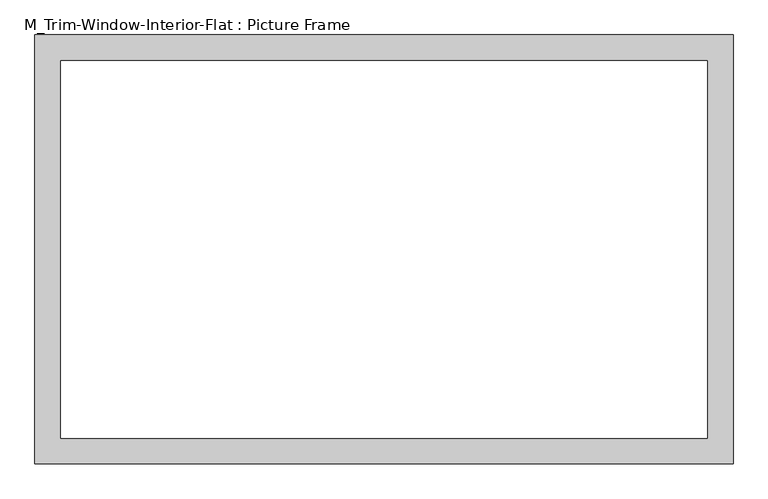
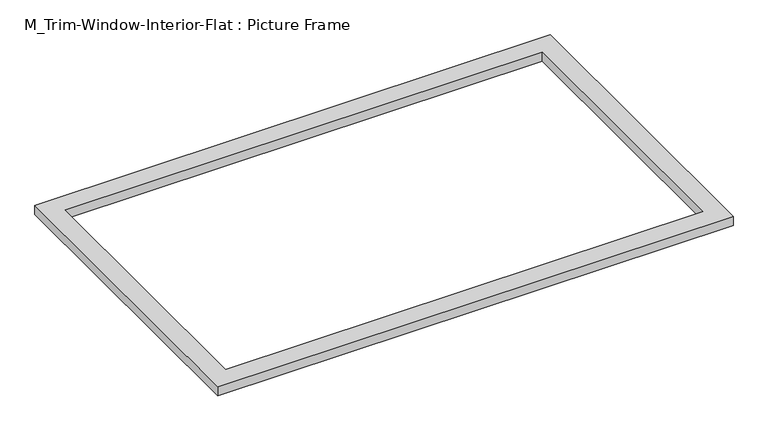
"""IFC4 building model written with IfcOpenShell, lengths in millimetres: proxy geometry, M_Trim-Window-Interior-Flat : Picture Frame."""

from ifc_helpers import new_model, si_unit, origin, origin_with_axes, place, context, project, spatial, polyline, outline, extrude, source, transform, mapped, element, save


def m_trim_window_interior_flat_picture_frame_90bf1a90(model_context):
    return source(origin(), model_context, "Body", "SweptSolid", [
        extrude(outline(polyline([(809.3, 47.3), (809.3, -947.3), (-809.3, -947.3), (-809.3, 47.3), (809.3, 47.3)]), holes=[polyline([(749.3, -12.7), (-749.3, -12.7), (-749.3, -887.3), (749.3, -887.3), (749.3, -12.7)])]), origin_with_axes(), (0.0, 0.0, 1.0), 30.0),
    ])


if __name__ == "__main__":
    model = new_model("IFC4")
    model_context = context("Model", 3, world=origin())
    ifc_project = project(units=[si_unit("LENGTHUNIT", "METRE", prefix="MILLI")], contexts=[model_context])
    site = spatial("IfcSite", under=ifc_project)
    building = spatial("IfcBuilding", under=site)
    placement = place(None, origin())
    m_trim_window_interior_flat_picture_frame_shape = m_trim_window_interior_flat_picture_frame_90bf1a90(model_context)
    element("IfcBuildingElementProxy", 1, Name="M_Trim-Window-Interior-Flat : Picture Frame", ObjectType="M_Trim-Window-Interior-Flat : Picture Frame", at=placement, inside=building, context=model_context, shape_type="MappedRepresentation", body=[
        mapped(m_trim_window_interior_flat_picture_frame_shape, transform((0.0, 0.0, 0.0), x_axis=(1.0, 0.0, 0.0), y_axis=(0.0, 1.0, 0.0), z_axis=(0.0, 0.0, 1.0))),
    ])
    save(model, "model.ifc")

# Revit data of these elements
# Type "M_Trim-Window-Interior-Flat : Picture Frame"
#   Trim Thickness_Picture Frame = 0' - 1.1811"
#   Trim Width = 0' - 2.3622"
#   Trim Thickness_with Sill = 0' - 0.7874"
#   Sill Thickness = 0' - 1.1811"
#   Opening Width [instance default] = 1' - 11.62205"
#   Opening Height [instance default] = 2' - 11.43307"
#   Default Elevation = 3' - 11.24409"
#   Sill = no
#   Picture Frame = yes
#   Trim Material [instance default] = none
# Element 1 (IfcBuildingElementProxy, "M_Trim-Window-Interior-Flat : Picture Frame")
#   Opening Width = 5' - 0"
#   Trim Material = Wood - Stained
#   Materials on its faces: "Wood - Stained"
# Materials
#   "Wood - Stained": class "Wood", colour RGB 224 178 126, transparency 0, Cost = 0
